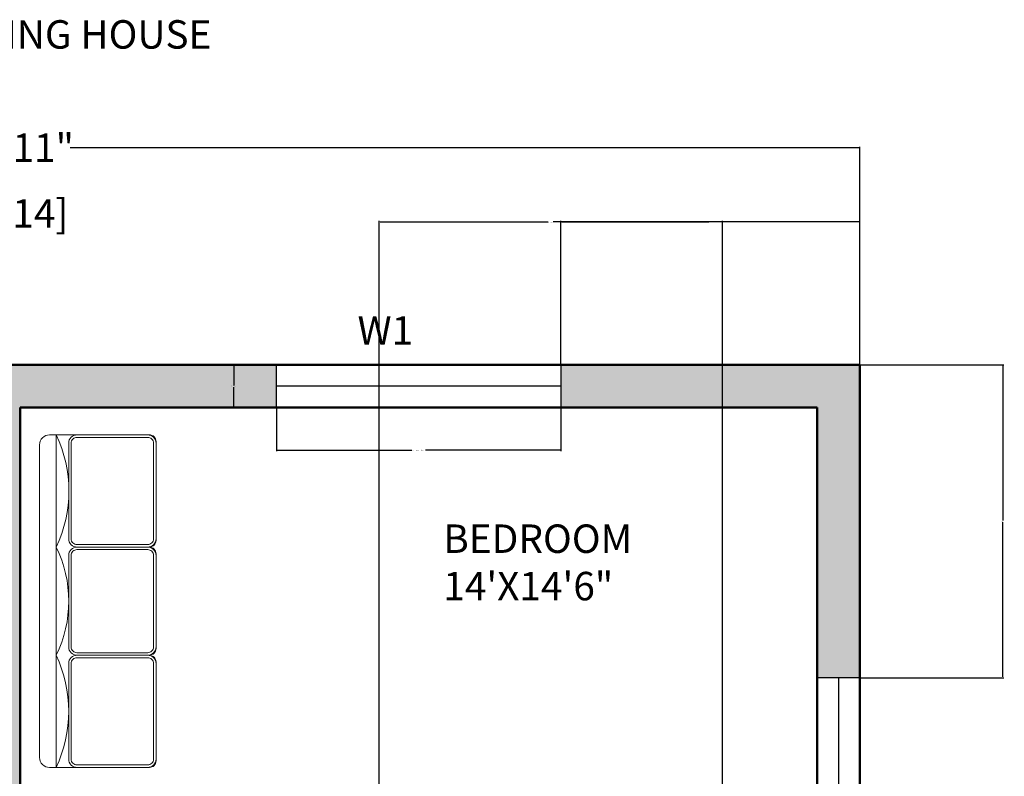
# Model space of a CAD drawing. Units: inches. Extents: x -15 to 420, y -514 to 86.
# Tile 8 of 8: x 212 to 420, y -74 to 86. Entities that reach past the tile are written whole.
import ezdxf

# ---------------------------------------------------------------- set-up
doc = ezdxf.new("R2010")
doc.units = ezdxf.units.IN
doc.header["$MEASUREMENT"] = 0
for name, color, linetype, lineweight in [('A-ANNO-DIMS', 2, 'Continuous', 18), ('A-ANNO-TEXT', 7, 'Continuous', 18), ('A-AREA-IDEN', 7, 'Continuous', 25), ('A-FURN', 8, 'Continuous', 18), ('A-GLAZ', 41, 'Continuous', 25), ('A-WALL', 7, 'Continuous', 50), ('A-WALL-PATT', 8, 'Continuous', 13)]:
    doc.layers.add(name, color=color, linetype=linetype, lineweight=lineweight)
doc.styles.get("Standard").update_dxf_attribs({"font": 'arial.ttf'})
doc.dimstyles.get("Standard").update_dxf_attribs({"dimtxt": 0.18, "dimasz": 0.18, "dimexe": 0.18, "dimexo": 0.0625, "dimgap": 0.09, "dimtad": 0, "dimtih": 1, "dimtoh": 1, "dimdec": 0, "dimzin": 0, "dimdsep": 46, "dimlunit": 3, "dimtxsty": 'Standard', "dimcen": 0.09, "dimadec": 0, "dimazin": 0, "dimtfac": 1, "dimtdec": 0, "dimtofl": 0, "dimtmove": 0, "dimatfit": 3, "dimfxl": 1, "dimtolj": 1, "dimtzin": 0, "dimarcsym": 0})

# ---------------------------------------------------------------- blocks, each defined once
blk = doc.blocks.new('*D1')
at = {"layer": 'A-ANNO-DIMS', "color": 0, "lineweight": -2, "transparency": 16777216}
for p, q in [((30.92, 13.18), (30.92, 59.13)), ((31.1, 58.95), (197.4, 58.95)), ((389.24, 58.95), (222.95, 58.95)), ((389.42, 13.18), (389.42, 59.13))]:
    blk.add_line(p, q, dxfattribs=at)
at = {"layer": 'A-ANNO-DIMS', "color": 0, "transparency": 16777216}
for points in [[(31.1, 58.98), (31.1, 58.92), (30.92, 58.95)], [(389.24, 58.98), (389.24, 58.92), (389.42, 58.95)]]:
    blk.add_solid(points, dxfattribs=at)
at = {"layer": 'Defpoints', "color": 0, "transparency": 16777216}
for p in [(389.42, 58.95), (30.92, 13.12), (389.42, 13.12)]:
    blk.add_point(p, dxfattribs=at)
at = {"layer": 'A-ANNO-DIMS', "color": 0, "transparency": 16777216, "insert": (210.17, 58.95), "char_height": 6, "attachment_point": 5}
blk.add_mtext('\\A1;29\'-11"', dxfattribs=at)
blk = doc.blocks.new('WIN-W1-60IN')
for p, q in [((0, 60), (0, 0)), ((4.5, 60), (4.5, 0)), ((9, 0), (9, 60))]:
    blk.add_line(p, q)
blk = doc.blocks.new('*D17')
at = {"layer": 'A-ANNO-DIMS', "color": 0, "lineweight": -2, "transparency": 16777216}
for p, q in [((266.42, 4.06), (266.42, -5.06)), ((326.42, 4.06), (326.42, -5.06)), ((266.6, -4.88), (294.97, -4.88)), ((326.24, -4.88), (297.88, -4.88))]:
    blk.add_line(p, q, dxfattribs=at)
at = {"layer": 'A-ANNO-DIMS', "color": 0, "transparency": 16777216}
for points in [[(266.6, -4.85), (266.6, -4.91), (266.42, -4.88)], [(326.24, -4.85), (326.24, -4.91), (326.42, -4.88)]]:
    blk.add_solid(points, dxfattribs=at)
at = {"layer": 'Defpoints', "color": 0, "transparency": 16777216}
for p in [(266.42, 4.12), (326.42, 4.12), (326.42, -4.88)]:
    blk.add_point(p, dxfattribs=at)
at = {"layer": 'A-ANNO-DIMS', "color": 0, "transparency": 16777216, "insert": (296.42, -4.88), "char_height": 0.18, "attachment_point": 5}
blk.add_mtext('\\A1;WINDOW W1 5\'-0" TYP.', dxfattribs=at)
blk = doc.blocks.new('*D18')
at = {"layer": 'A-ANNO-DIMS', "color": 0, "lineweight": -2, "transparency": 16777216}
for p, q in [((266.36, 13.12), (257.24, 13.12)), ((257.42, 12.94), (257.42, 8.8)), ((257.42, 4.3), (257.42, 8.44)), ((266.36, 4.12), (257.24, 4.12))]:
    blk.add_line(p, q, dxfattribs=at)
at = {"layer": 'A-ANNO-DIMS', "color": 0, "transparency": 16777216}
for points in [[(257.39, 12.94), (257.45, 12.94), (257.42, 13.12)], [(257.39, 4.3), (257.45, 4.3), (257.42, 4.12)]]:
    blk.add_solid(points, dxfattribs=at)
at = {"layer": 'Defpoints', "color": 0, "transparency": 16777216}
for p in [(266.42, 13.12), (257.42, 4.12), (266.42, 4.12)]:
    blk.add_point(p, dxfattribs=at)
at = {"layer": 'A-ANNO-DIMS', "color": 0, "transparency": 16777216, "insert": (257.42, 8.62), "char_height": 0.18, "attachment_point": 5}
blk.add_mtext('\\A1;0\'-9" TYP.', dxfattribs=at)
blk = doc.blocks.new('*D60')
at = {"layer": 'A-ANNO-DIMS', "color": 0, "lineweight": -2, "transparency": 16777216}
for p, q in [((326.42, 13.18), (326.42, 43.5)), ((326.6, 43.32), (357.6, 43.32)), ((389.24, 43.32), (358.25, 43.32)), ((389.42, 13.18), (389.42, 43.5))]:
    blk.add_line(p, q, dxfattribs=at)
at = {"layer": 'A-ANNO-DIMS', "color": 0, "transparency": 16777216}
for points in [[(326.6, 43.35), (326.6, 43.29), (326.42, 43.32)], [(389.24, 43.35), (389.24, 43.29), (389.42, 43.32)]]:
    blk.add_solid(points, dxfattribs=at)
at = {"layer": 'Defpoints', "color": 0, "transparency": 16777216}
for p in [(389.42, 43.32), (326.42, 13.12), (389.42, 13.12)]:
    blk.add_point(p, dxfattribs=at)
at = {"layer": 'A-ANNO-DIMS', "color": 0, "transparency": 16777216, "insert": (357.92, 43.32), "char_height": 0.18, "attachment_point": 5}
blk.add_mtext('\\A1;5\'-3"', dxfattribs=at)
blk = doc.blocks.new('*D61')
at = {"layer": 'A-ANNO-DIMS', "color": 0, "lineweight": -2, "transparency": 16777216}
for p, q in [((389.49, 13.12), (419.8, 13.12)), ((419.62, 12.94), (419.62, -19.7)), ((419.62, -52.7), (419.62, -20.06)), ((389.49, -52.88), (419.8, -52.88))]:
    blk.add_line(p, q, dxfattribs=at)
at = {"layer": 'A-ANNO-DIMS', "color": 0, "transparency": 16777216}
for points in [[(419.59, 12.94), (419.65, 12.94), (419.62, 13.12)], [(419.59, -52.7), (419.65, -52.7), (419.62, -52.88)]]:
    blk.add_solid(points, dxfattribs=at)
at = {"layer": 'Defpoints', "color": 0, "transparency": 16777216}
for p in [(389.42, 13.12), (419.62, 13.12), (389.42, -52.88)]:
    blk.add_point(p, dxfattribs=at)
at = {"layer": 'A-ANNO-DIMS', "color": 0, "transparency": 16777216, "insert": (419.62, -19.88), "char_height": 0.18, "attachment_point": 5}
blk.add_mtext('\\A1;5\'-6"', dxfattribs=at)
blk = doc.blocks.new('*D70')
at = {"layer": 'A-ANNO-DIMS', "color": 0, "lineweight": -2, "transparency": 16777216}
for p, q in [((288.09, -76.72), (288.09, 43.5)), ((288.27, 43.32), (323.74, 43.32)), ((360.28, 43.32), (324.81, 43.32)), ((360.46, -76.72), (360.46, 43.5))]:
    blk.add_line(p, q, dxfattribs=at)
at = {"layer": 'A-ANNO-DIMS', "color": 0, "transparency": 16777216}
for points in [[(288.27, 43.35), (288.27, 43.29), (288.09, 43.32)], [(360.28, 43.35), (360.28, 43.29), (360.46, 43.32)]]:
    blk.add_solid(points, dxfattribs=at)
at = {"layer": 'Defpoints', "color": 0, "transparency": 16777216}
for p in [(360.46, 43.32), (288.09, -76.78), (360.46, -76.78)]:
    blk.add_point(p, dxfattribs=at)
at = {"layer": 'A-ANNO-DIMS', "color": 0, "transparency": 16777216, "insert": (324.27, 43.32), "char_height": 0.18, "attachment_point": 5}
blk.add_mtext('\\A1;6\'-0 1/2"', dxfattribs=at)

msp = doc.modelspace()

# ---------------------------------------------------------------- hatches: boundary and pattern name
at = {"layer": 'A-WALL-PATT'}
h = msp.add_hatch(color=256, dxfattribs=at)
h.dxf.hatch_style = 1
h.paths.add_polyline_path([(266.67, -454.88), (240.92, -454.88), (240.92, -330.38), (236.42, -330.38), (236.42, -454.88), (218.42, -454.88), (218.42, -463.88), (266.67, -463.88)])
h.paths.add_polyline_path([(158.42, -454.88), (140.42, -454.88), (140.42, -394.88), (135.92, -394.88), (135.92, -454.88), (39.92, -454.88), (39.92, -412.88), (30.92, -412.88), (30.92, -463.88), (158.42, -463.88)])
h.paths.add_polyline_path([(39.92, -334.88), (135.92, -334.88), (135.92, -357.15), (140.42, -357.15), (140.42, -334.88), (173.95, -334.88), (173.95, -330.38), (39.92, -330.38), (39.92, -250.88), (155.51, -250.88), (155.51, -246.38), (140.42, -246.38), (140.42, -205.38), (138.17, -205.38), (135.92, -205.38), (135.92, -246.38), (39.92, -246.38), (39.92, -222.38), (30.92, -222.38), (30.92, -376.88), (39.92, -376.88)])
h.paths.add_polyline_path([(389.42, -382.88), (380.42, -382.88), (380.42, -454.88), (380.42, -463.88), (389.42, -463.88)])
h.paths.add_polyline_path([(352.42, -459.38), (352.42, -454.88), (326.67, -454.88), (326.67, -463.88), (352.42, -463.88)])
h.paths.add_polyline_path([(176.92, -169.88), (39.92, -169.88), (39.92, -112.88), (30.92, -112.88), (30.92, -198.38), (39.92, -198.38), (39.92, -174.38), (135.92, -174.38), (135.92, -177.38), (140.42, -177.38), (140.42, -174.38), (176.92, -174.38), (176.92, -172.13)])
h.paths.add_polyline_path([(39.92, 4.12), (93.92, 4.12), (93.92, 13.12), (30.92, 13.12), (30.92, -52.88), (39.92, -52.88)])
h.paths.add_polyline_path([(266.42, 13.12), (153.92, 13.12), (153.92, 4.12), (207.92, 4.12), (207.92, -169.88), (204.92, -169.88), (204.92, -174.38), (215.42, -174.38), (215.42, -169.88), (212.42, -169.88), (212.42, 4.12), (266.42, 4.12)])
h.paths.add_polyline_path([(389.42, 13.12), (326.42, 13.12), (326.42, 4.12), (380.42, 4.12), (380.42, -52.88), (389.42, -52.88)])
h.paths.add_polyline_path([(389.42, -112.88), (380.42, -112.88), (380.42, -169.88), (377.42, -169.88), (377.42, -174.38), (380.42, -174.38), (380.42, -198.38), (389.42, -198.38)])
h.paths.add_polyline_path([(349.42, -172.13), (349.42, -169.88), (243.42, -169.88), (243.42, -172.13), (243.42, -174.38), (279.92, -174.38), (279.92, -250.88), (380.42, -250.88), (380.42, -322.88), (389.42, -322.88), (389.42, -222.38), (380.42, -222.38), (380.42, -246.38), (284.42, -246.38), (284.42, -174.38), (349.42, -174.38)])

# ---------------------------------------------------------------- linework, layer by layer
at = {"layer": 'A-FURN', "ltscale": 0.03}
msp.add_lwpolyline([(241.05, -49.53), (241.05, -70.38, -0.414214), (239.64, -71.79), (218.6, -71.79, -0.414214), (216.49, -69.68), (216.49, -3.73, -0.414214), (218.6, -1.63), (239.64, -1.63, -0.414214), (241.05, -3.03), (241.05, -23.89, -0.414214), (239.64, -25.29, 1), (239.64, -25.32, -0.414214), (241.05, -26.73), (241.05, -46.69, -0.414214), (239.64, -48.09, 1), (239.64, -48.13, -0.414214)], format="xyb", close=True, dxfattribs=at)
at = {"layer": 'A-FURN'}
msp.add_lwpolyline([(220, -71.79), (220, -1.63)], dxfattribs=at)
for points in [[(239.29, -25.31), (224.38, -25.31, -0.414214), (222.63, -23.55), (222.63, -3.38, -0.414214), (224.38, -1.63), (239.29, -1.63, -0.414214), (241.05, -3.38), (241.05, -23.55, -0.414214)], [(239.29, -24.78), (224.38, -24.78, -0.414214), (223.16, -23.55), (223.16, -3.38, -0.414214), (224.38, -2.15), (239.29, -2.15, -0.414214), (240.52, -3.38), (240.52, -23.55, -0.414214)], [(239.29, -25.31), (224.38, -25.31, 0.414214), (222.63, -27.06), (222.63, -46.35, 0.414214), (224.38, -48.11), (239.29, -48.11, 0.414214), (241.05, -46.35), (241.05, -27.06, 0.414214)], [(239.29, -25.83), (224.38, -25.83, 0.414214), (223.16, -27.06), (223.16, -46.35, 0.414214), (224.38, -47.58), (239.29, -47.58, 0.414214), (240.52, -46.35), (240.52, -27.06, 0.414214)], [(239.29, -71.79), (224.38, -71.79, -0.414214), (222.63, -70.03), (222.63, -49.86, -0.414214), (224.38, -48.11), (239.29, -48.11, -0.414214), (241.05, -49.86), (241.05, -70.03, -0.414214)], [(239.29, -71.26), (224.38, -71.26, -0.414214), (223.16, -70.03), (223.16, -49.86, -0.414214), (224.38, -48.63), (239.29, -48.63, -0.414214), (240.52, -49.86), (240.52, -70.03, -0.414214)]]:
    msp.add_lwpolyline(points, format="xyb", close=True, dxfattribs=at)
for centre, radius, start, end in [((195.01, -13.47), 27.66, 334.6538, 25.3462), ((196.76, -36.71), 25.89, 333.869, 26.131), ((194.71, -59.95), 27.92, 334.9106, 25.0894)]:
    msp.add_arc(centre, radius, start, end, dxfattribs=at)
at = {"layer": 'A-GLAZ'}
for p, q in [((266.42, 4.12), (266.42, 13.12)), ((326.42, 13.12), (326.42, 4.12)), ((389.42, -52.88), (380.42, -52.88))]:
    msp.add_line(p, q, dxfattribs=at)
at = {"layer": 'A-WALL'}
for p, q in [((30.92, 13.12), (389.42, 13.12)), ((389.42, 13.12), (389.42, -463.88)), ((212.42, 4.12), (212.42, -169.88)), ((212.42, 4.12), (380.42, 4.12)), ((380.42, 4.12), (380.42, -169.88))]:
    msp.add_line(p, q, dxfattribs=at)

# ---------------------------------------------------------------- block references
at = {"layer": 'A-GLAZ', "rotation": 270}
msp.add_blockref('WIN-W1-60IN', (266.43, 13.12), dxfattribs=at)
at = {"layer": 'A-GLAZ'}
msp.add_blockref('WIN-W1-60IN', (380.43, -112.88), dxfattribs=at)

# ---------------------------------------------------------------- texts
at = {"layer": 'A-ANNO-DIMS', "insert": (201.17, 48.09), "char_height": 6, "attachment_point": 1}
msp.add_mtext('[9.14]', dxfattribs=at)
at = {"layer": 'A-ANNO-TEXT', "char_height": 6, "attachment_point": 1}
for s, insert in [('EAST FACING HOUSE', (173.17, 85.85)), ('W1', (283.53, 23.4))]:
    msp.add_mtext(s, dxfattribs=dict(at, insert=insert))
at = {"layer": 'A-AREA-IDEN', "insert": (301.61, -20.53), "char_height": 6, "attachment_point": 1}
msp.add_mtext('BEDROOM\\P14\'X14\'6"', dxfattribs=at)

# ---------------------------------------------------------------- dimensions: what is measured, and where the dimension line sits
at = {"layer": 'A-ANNO-DIMS'}
for base, p1, p2, override, picture, middle in [((389.42485788, 58.94777598), (30.92485788, 13.12050654), (389.42485788, 13.12050654), {"dimtxt": 6, "dimclrd": 0, "dimclre": 0, "dimclrt": 0}, '*D1', (210.17485788, 58.94777598)), ((360.46, 43.32), (288.09, -76.78), (360.46, -76.78), {"dimdec": 1, "dimlfac": 1, "dimrnd": 0, "dimzin": 1, "dimdsep": 46, "dimlunit": 4, "dimfrac": 2}, '*D70', (324.27, 43.32)), ((389.42, 43.32), (326.42, 13.12), (389.42, 13.12), {"dimdec": 1, "dimlfac": 1, "dimrnd": 0, "dimzin": 1, "dimdsep": 46, "dimlunit": 4, "dimfrac": 2}, '*D60', (357.92, 43.32))]:
    dim = msp.add_linear_dim(base=base, p1=p1, p2=p2, dimstyle='Standard', override=override, dxfattribs=at)
    dim.commit()
    dim.dimension.update_dxf_attribs({"geometry": picture, "text_midpoint": middle})
dim = msp.add_linear_dim(base=(257.42, 4.12), p1=(266.42, 13.12), p2=(266.42, 4.12), angle=270, text='<> TYP.', dimstyle='Standard', override={"dimdec": 1, "dimlfac": 1, "dimrnd": 0, "dimzin": 1, "dimdsep": 46, "dimlunit": 4, "dimfrac": 2}, dxfattribs=at)
dim.commit()
dim.dimension.update_dxf_attribs({"geometry": '*D18', "text_midpoint": (257.42, 8.62)})
dim = msp.add_linear_dim(base=(419.62, 13.12), p1=(389.42, -52.88), p2=(389.42, 13.12), angle=90, dimstyle='Standard', override={"dimdec": 1, "dimlfac": 1, "dimrnd": 0, "dimzin": 1, "dimdsep": 46, "dimlunit": 4, "dimfrac": 2}, dxfattribs=at)
dim.commit()
dim.dimension.update_dxf_attribs({"geometry": '*D61', "text_midpoint": (419.62, -19.88)})
dim = msp.add_linear_dim(base=(326.42, -4.88), p1=(266.42, 4.12), p2=(326.42, 4.12), text='WINDOW W1 <> TYP.', dimstyle='Standard', override={"dimdec": 1, "dimlfac": 1, "dimrnd": 0, "dimzin": 1, "dimdsep": 46, "dimlunit": 4, "dimfrac": 2}, dxfattribs=at)
dim.commit()
dim.dimension.update_dxf_attribs({"geometry": '*D17', "text_midpoint": (296.42, -4.88)})

doc.saveas('drawing.dxf')
